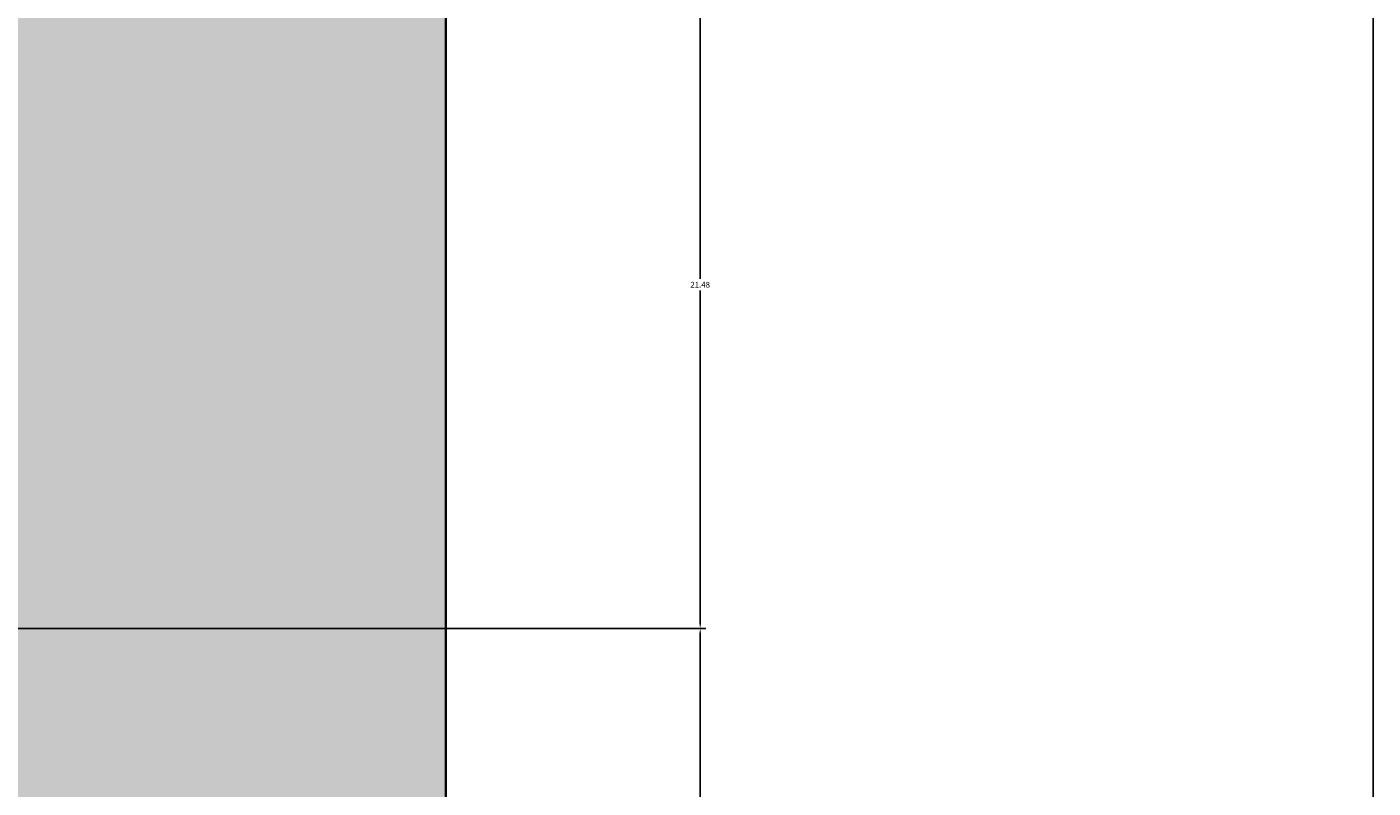
# Model space of a CAD drawing. Units: inches. Extents: x 4508 to 4723, y 847 to 1020.
# Tile 25 of 32: x 4681 to 4723, y 910 to 933. Entities that reach past the tile are written whole.
import ezdxf

# ---------------------------------------------------------------- set-up
doc = ezdxf.new("R2010")
doc.units = ezdxf.units.IN
for name, color, linetype, lineweight in [('A-ANNO-DIMS', 2, 'Continuous', 18), ('A-ANNO-TTLB', 7, 'Continuous', 25), ('A-WALL', 7, 'Continuous', 35), ('A-WALL-PATT', 254, 'Continuous', 13)]:
    doc.layers.add(name, color=color, linetype=linetype, lineweight=lineweight)
doc.styles.get("Standard").update_dxf_attribs({"font": 'arial.ttf'})
doc.dimstyles.get("Standard").update_dxf_attribs({"dimtxt": 0.18, "dimasz": 0.18, "dimexe": 0.18, "dimexo": 0.0625, "dimgap": 0.09, "dimtad": 0, "dimtih": 1, "dimtoh": 1, "dimdec": 4, "dimzin": 0, "dimdsep": 46, "dimtxsty": 'Standard', "dimcen": 0.09, "dimadec": 0, "dimazin": 0, "dimtfac": 1, "dimtdec": 4, "dimtofl": 0, "dimtmove": 0, "dimatfit": 3, "dimfxl": 1, "dimtolj": 1, "dimtzin": 0, "dimarcsym": 0})

# ---------------------------------------------------------------- blocks, each defined once
blk = doc.blocks.new('*D13')
at = {"layer": 'A-ANNO-DIMS', "color": 0, "lineweight": -2, "transparency": 16777216}
for p, q in [((4669.325, 973.916), (4669.325, 866.617)), ((4689.994, 874.684), (4689.994, 866.617)), ((4669.505, 866.797), (4679.264, 866.797)), ((4689.814, 866.797), (4680.054, 866.797))]:
    blk.add_line(p, q, dxfattribs=at)
at = {"layer": 'A-ANNO-DIMS', "color": 0, "lineweight": 9, "transparency": 16777216}
for points in [[(4669.505, 866.827), (4669.505, 866.767), (4669.325, 866.797)], [(4689.814, 866.827), (4689.814, 866.767), (4689.994, 866.797)]]:
    blk.add_solid(points, dxfattribs=at)
at = {"layer": 'Defpoints', "color": 0, "lineweight": 9, "transparency": 16777216}
for p in [(4669.325, 973.978), (4689.994, 874.747), (4689.994, 866.797)]:
    blk.add_point(p, dxfattribs=at)
at = {"layer": 'A-ANNO-DIMS', "color": 0, "transparency": 16777216, "insert": (4679.659, 866.797), "char_height": 0.18, "attachment_point": 5}
blk.add_mtext('\\A1;20.67', dxfattribs=at)
blk = doc.blocks.new('*D19')
at = {"layer": 'A-ANNO-DIMS', "color": 0, "lineweight": -2, "transparency": 16777216}
for p, q in [((4662.233, 914.641), (4702.124, 914.641)), ((4701.944, 914.461), (4701.944, 908.376)), ((4701.944, 901.927), (4701.944, 908.012)), ((4671.119, 901.747), (4702.124, 901.747))]:
    blk.add_line(p, q, dxfattribs=at)
at = {"layer": 'A-ANNO-DIMS', "color": 0, "lineweight": 9, "transparency": 16777216}
for points in [[(4701.914, 914.461), (4701.974, 914.461), (4701.944, 914.641)], [(4701.914, 901.927), (4701.974, 901.927), (4701.944, 901.747)]]:
    blk.add_solid(points, dxfattribs=at)
at = {"layer": 'Defpoints', "color": 0, "lineweight": 9, "transparency": 16777216}
for p in [(4662.171, 914.641), (4701.944, 914.641), (4671.056, 901.747)]:
    blk.add_point(p, dxfattribs=at)
at = {"layer": 'A-ANNO-DIMS', "color": 0, "transparency": 16777216, "insert": (4701.944, 908.194), "char_height": 0.18, "attachment_point": 5}
blk.add_mtext('\\A1;12.894', dxfattribs=at)
blk = doc.blocks.new('*D20')
at = {"layer": 'A-ANNO-DIMS', "color": 0, "lineweight": -2, "transparency": 16777216}
for p, q in [((4667.324, 936.122), (4702.124, 936.122)), ((4701.944, 935.942), (4701.944, 925.563)), ((4701.944, 914.821), (4701.944, 925.2)), ((4662.233, 914.641), (4702.124, 914.641))]:
    blk.add_line(p, q, dxfattribs=at)
at = {"layer": 'A-ANNO-DIMS', "color": 0, "lineweight": 9, "transparency": 16777216}
for points in [[(4701.914, 935.942), (4701.974, 935.942), (4701.944, 936.122)], [(4701.914, 914.821), (4701.974, 914.821), (4701.944, 914.641)]]:
    blk.add_solid(points, dxfattribs=at)
at = {"layer": 'Defpoints', "color": 0, "lineweight": 9, "transparency": 16777216}
for p in [(4667.262, 936.122), (4701.944, 936.122), (4662.171, 914.641)]:
    blk.add_point(p, dxfattribs=at)
at = {"layer": 'A-ANNO-DIMS', "color": 0, "transparency": 16777216, "insert": (4701.944, 925.381), "char_height": 0.18, "attachment_point": 5}
blk.add_mtext('\\A1;21.48', dxfattribs=at)

msp = doc.modelspace()

# ---------------------------------------------------------------- hatches: boundary and pattern name
at = {"layer": 'A-WALL-PATT', "transparency": 33554508}
h = msp.add_hatch(color=256, dxfattribs=at)
h.dxf.hatch_style = 1
h.paths.add_polyline_path([(4661.6706, 954.043, -0.3739004), (4658.5765, 957.6021, -1), (4665.7646, 957.6021, -0.3739004), (4662.6706, 954.043), (4662.6706, 944.4021, -0.2114781), (4670.3062, 945.0869), (4670.3062, 968.0592, -0.4632086), (4663.3246, 973.9783, -0.4632086), (4670.3062, 979.8975), (4670.3062, 994.7469), (4588.9938, 994.7469), (4588.9938, 904.7469), (4657.9938, 904.7469), (4657.9938, 886.7469), (4549.9938, 886.7469), (4549.9938, 878.7469), (4693.9938, 878.7469), (4693.9938, 994.7469), (4671.8062, 994.7469), (4671.8062, 979.4411, -0.2941682), (4675.3246, 973.9783, -0.2941682), (4671.8062, 968.5156), (4671.8062, 944.4278, -0.2741114), (4676.7298, 936.1217, -0.2741114), (4671.8062, 927.8155), (4671.8062, 907.6998, -0.3779645), (4677.0562, 901.7469, -0.3779645), (4671.8062, 895.7939), (4671.8062, 883.7469), (4670.3062, 883.7469), (4670.3062, 895.7939, -0.3779645), (4665.0562, 901.7469, -0.3779645), (4670.3062, 907.6998), (4670.3062, 927.1564, -0.2114781), (4662.6706, 927.8412), (4662.6706, 918.2003, -0.3739004), (4665.7646, 914.6412, -1), (4658.5765, 914.6412, -0.3739004), (4661.6706, 918.2003), (4661.6706, 928.4807, -0.2391825), (4657.7936, 936.1217, -0.2391825), (4661.6706, 943.7626)])

# ---------------------------------------------------------------- linework, layer by layer
at = {"layer": 'A-ANNO-TTLB'}
msp.add_lwpolyline([(4508.3867, 1019.9118), (4722.9774, 1019.9118), (4722.9774, 846.9535), (4508.3867, 846.9535)], close=True, dxfattribs=at)
at = {"layer": 'A-WALL'}
msp.add_line((4693.9938, 994.7469), (4693.9938, 874.7469), dxfattribs=at)

# ---------------------------------------------------------------- dimensions: what is measured, and where the dimension line sits
at = {"layer": 'A-ANNO-DIMS'}
dim = msp.add_linear_dim(base=(4689.9938, 866.7969), p1=(4669.3246, 973.9783), p2=(4689.9938, 874.7469), dimstyle='Standard', override={"dimdec": 2, "dimlfac": 1, "dimrnd": 0, "dimzin": 0, "dimdsep": 46, "dimlunit": 2}, dxfattribs=at)
dim.commit()
dim.dimension.update_dxf_attribs({"geometry": '*D13', "text_midpoint": (4679.6592, 866.7969)})
for base, p1, p2, override, picture, middle in [((4701.9438, 936.1217), (4662.1706, 914.6412), (4667.2617, 936.1217), {"dimdec": 2, "dimlfac": 1, "dimrnd": 0, "dimzin": 0, "dimdsep": 46, "dimlunit": 2}, '*D20', (4701.9438, 925.3814)), ((4701.9438, 914.6412), (4671.0562, 901.7469), (4662.1706, 914.6412), {"dimdec": 3, "dimlfac": 1, "dimrnd": 0, "dimzin": 0, "dimdsep": 46, "dimlunit": 2}, '*D19', (4701.9438, 908.1941))]:
    dim = msp.add_linear_dim(base=base, p1=p1, p2=p2, angle=90, dimstyle='Standard', override=override, dxfattribs=at)
    dim.commit()
    dim.dimension.update_dxf_attribs({"geometry": picture, "text_midpoint": middle})

doc.saveas('drawing.dxf')
